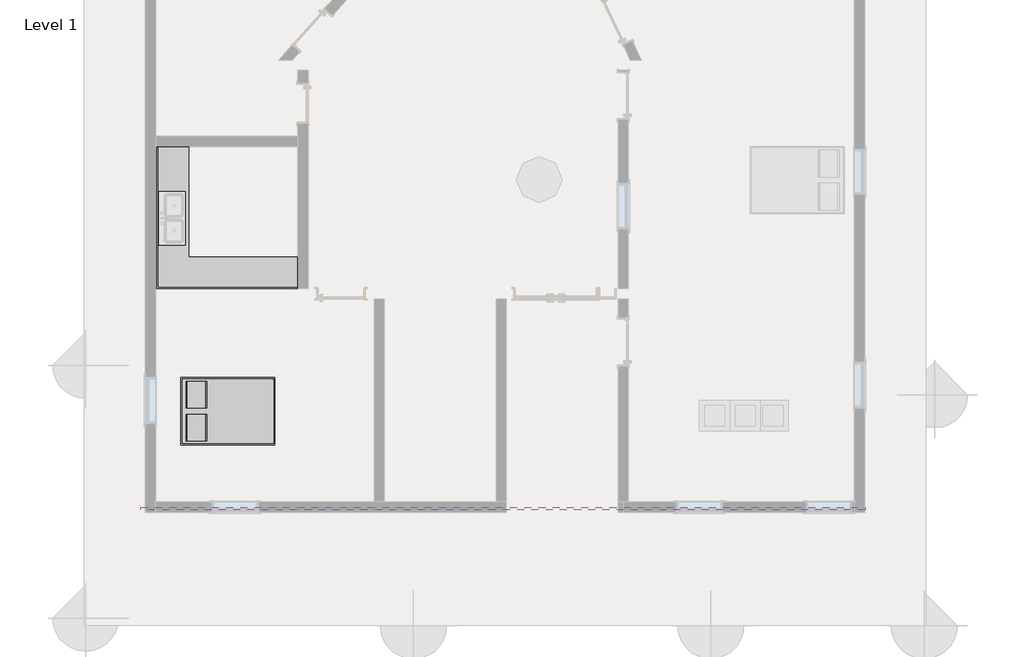
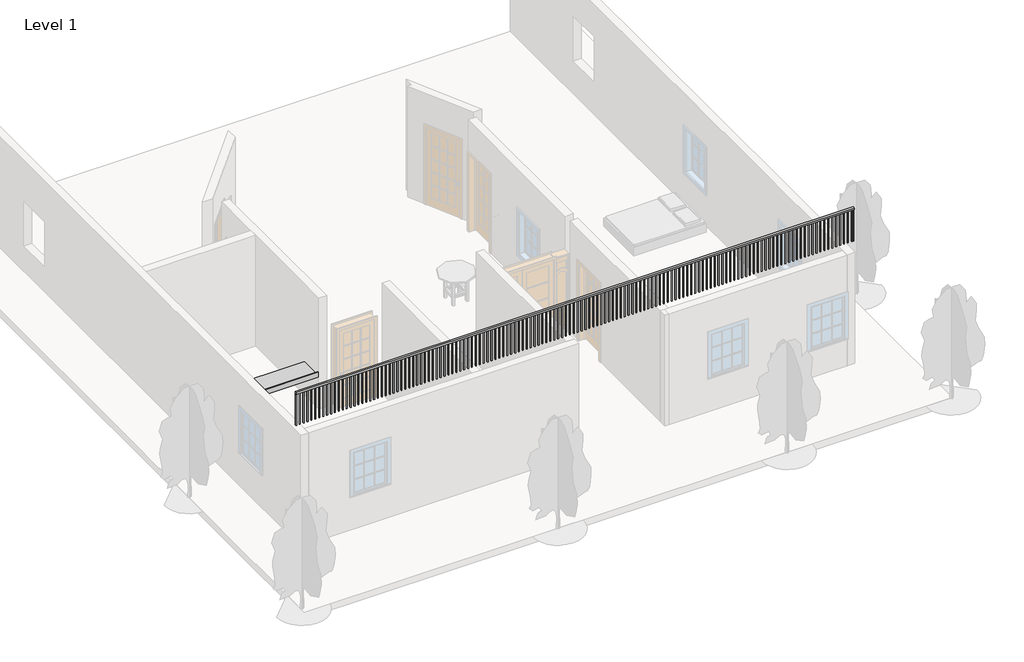
# One storey, part 2 of 3: 2 furniture elements, 1 railing.
"""IFC4 building model written with IfcOpenShell, lengths in millimetres."""

from ifc_helpers import new_model, si_unit, frame, origin, place, context, project, spatial, polyline, outline, extrude, transform, mapped, element, save
from components import furniture_c8abb964, furniture_ce44b9f3

model = new_model("IFC4")

# Units and contexts
model_context = context("Model", 3, world=origin())
ifc_project = project(units=[si_unit("LENGTHUNIT", "METRE", prefix="MILLI")], contexts=[model_context])

# Site, building, storey
site = spatial("IfcSite", under=ifc_project)
building = spatial("IfcBuilding", under=site)
storey = spatial("IfcBuildingStorey", under=building, Name="Level 1", Elevation=0.0)

# Furniture
placement = place(None, origin())
furniture_shape = furniture_c8abb964(model_context)
element("IfcFurniture", 1, ObjectType="Bed-Box : Double 53\" x 74\"", at=placement, inside=storey, context=model_context, shape_type="MappedRepresentation", body=[
    mapped(furniture_shape, transform((-8121.5392959, 5074.7783356, 0.0), x_axis=(0.0, 1.0000000000000018, 0.0), y_axis=(-1.0000000000000018, 0.0, 0.0), z_axis=(0.0, 0.0, 1.0))),
])
furniture_2_shape = furniture_ce44b9f3(model_context)
element("IfcFurniture", 2, ObjectType="Counter Top-L Shaped w Sink.0001 : 24\" Depth", at=placement, inside=storey, context=model_context, shape_type="MappedRepresentation", body=[
    mapped(furniture_2_shape, transform((-9309.5097877, 9065.4930897, 0.0), x_axis=(0.0, 1.0, 0.0), y_axis=(-1.0, 0.0, 0.0), z_axis=(0.0, 0.0, 1.0))),
])

# Railing
element("IfcRailing", 3, ObjectType="Handrail - Rectangular", at=placement, inside=storey, context=model_context, shape_type="SweptSolid", body=[
    extrude(outline(polyline([(-9630.8642944, 3438.5335491), (-9630.8642944, 3489.3335491), (4847.1357056, 3489.3335491), (4847.1357056, 3438.5335491), (-9630.8642944, 3438.5335491)])), frame((0.0, 0.0, 4185.9398438), z_axis=(0.0, 0.0, 1.0), x_axis=(1.0, 0.0, 0.0)), (0.0, 0.0, 1.0), 50.8),
    extrude(outline(polyline([(4786.8107056, 3454.4085491), (4786.8107056, 3473.4585491), (4805.8607056, 3473.4585491), (4805.8607056, 3454.4085491), (4786.8107056, 3454.4085491)])), frame((0.0, 0.0, 3322.3398438), z_axis=(0.0, 0.0, 1.0), x_axis=(1.0, 0.0, 0.0)), (0.0, 0.0, 1.0), 863.6),
    extrude(outline(polyline([(4685.2107056, 3454.4085491), (4685.2107056, 3473.4585491), (4704.2607056, 3473.4585491), (4704.2607056, 3454.4085491), (4685.2107056, 3454.4085491)])), frame((0.0, 0.0, 3322.3398438), z_axis=(0.0, 0.0, 1.0), x_axis=(1.0, 0.0, 0.0)), (0.0, 0.0, 1.0), 863.6),
    extrude(outline(polyline([(4583.6107056, 3454.4085491), (4583.6107056, 3473.4585491), (4602.6607056, 3473.4585491), (4602.6607056, 3454.4085491), (4583.6107056, 3454.4085491)])), frame((0.0, 0.0, 3322.3398438), z_axis=(0.0, 0.0, 1.0), x_axis=(1.0, 0.0, 0.0)), (0.0, 0.0, 1.0), 863.6),
    extrude(outline(polyline([(4482.0107056, 3454.4085491), (4482.0107056, 3473.4585491), (4501.0607056, 3473.4585491), (4501.0607056, 3454.4085491), (4482.0107056, 3454.4085491)])), frame((0.0, 0.0, 3322.3398438), z_axis=(0.0, 0.0, 1.0), x_axis=(1.0, 0.0, 0.0)), (0.0, 0.0, 1.0), 863.6),
    extrude(outline(polyline([(4380.4107056, 3454.4085491), (4380.4107056, 3473.4585491), (4399.4607056, 3473.4585491), (4399.4607056, 3454.4085491), (4380.4107056, 3454.4085491)])), frame((0.0, 0.0, 3322.3398438), z_axis=(0.0, 0.0, 1.0), x_axis=(1.0, 0.0, 0.0)), (0.0, 0.0, 1.0), 863.6),
    extrude(outline(polyline([(4278.8107056, 3454.4085491), (4278.8107056, 3473.4585491), (4297.8607056, 3473.4585491), (4297.8607056, 3454.4085491), (4278.8107056, 3454.4085491)])), frame((0.0, 0.0, 3322.3398438), z_axis=(0.0, 0.0, 1.0), x_axis=(1.0, 0.0, 0.0)), (0.0, 0.0, 1.0), 863.6),
    extrude(outline(polyline([(4177.2107056, 3454.4085491), (4177.2107056, 3473.4585491), (4196.2607056, 3473.4585491), (4196.2607056, 3454.4085491), (4177.2107056, 3454.4085491)])), frame((0.0, 0.0, 3322.3398438), z_axis=(0.0, 0.0, 1.0), x_axis=(1.0, 0.0, 0.0)), (0.0, 0.0, 1.0), 863.6),
    extrude(outline(polyline([(4075.6107056, 3454.4085491), (4075.6107056, 3473.4585491), (4094.6607056, 3473.4585491), (4094.6607056, 3454.4085491), (4075.6107056, 3454.4085491)])), frame((0.0, 0.0, 3322.3398438), z_axis=(0.0, 0.0, 1.0), x_axis=(1.0, 0.0, 0.0)), (0.0, 0.0, 1.0), 863.6),
    extrude(outline(polyline([(3974.0107056, 3454.4085491), (3974.0107056, 3473.4585491), (3993.0607056, 3473.4585491), (3993.0607056, 3454.4085491), (3974.0107056, 3454.4085491)])), frame((0.0, 0.0, 3322.3398438), z_axis=(0.0, 0.0, 1.0), x_axis=(1.0, 0.0, 0.0)), (0.0, 0.0, 1.0), 863.6),
    extrude(outline(polyline([(3872.4107056, 3454.4085491), (3872.4107056, 3473.4585491), (3891.4607056, 3473.4585491), (3891.4607056, 3454.4085491), (3872.4107056, 3454.4085491)])), frame((0.0, 0.0, 3322.3398438), z_axis=(0.0, 0.0, 1.0), x_axis=(1.0, 0.0, 0.0)), (0.0, 0.0, 1.0), 863.6),
    extrude(outline(polyline([(3770.8107056, 3454.4085491), (3770.8107056, 3473.4585491), (3789.8607056, 3473.4585491), (3789.8607056, 3454.4085491), (3770.8107056, 3454.4085491)])), frame((0.0, 0.0, 3322.3398438), z_axis=(0.0, 0.0, 1.0), x_axis=(1.0, 0.0, 0.0)), (0.0, 0.0, 1.0), 863.6),
    extrude(outline(polyline([(3669.2107056, 3454.4085491), (3669.2107056, 3473.4585491), (3688.2607056, 3473.4585491), (3688.2607056, 3454.4085491), (3669.2107056, 3454.4085491)])), frame((0.0, 0.0, 3322.3398438), z_axis=(0.0, 0.0, 1.0), x_axis=(1.0, 0.0, 0.0)), (0.0, 0.0, 1.0), 863.6),
    extrude(outline(polyline([(3567.6107056, 3454.4085491), (3567.6107056, 3473.4585491), (3586.6607056, 3473.4585491), (3586.6607056, 3454.4085491), (3567.6107056, 3454.4085491)])), frame((0.0, 0.0, 3322.3398438), z_axis=(0.0, 0.0, 1.0), x_axis=(1.0, 0.0, 0.0)), (0.0, 0.0, 1.0), 863.6),
    extrude(outline(polyline([(3466.0107056, 3454.4085491), (3466.0107056, 3473.4585491), (3485.0607056, 3473.4585491), (3485.0607056, 3454.4085491), (3466.0107056, 3454.4085491)])), frame((0.0, 0.0, 3322.3398438), z_axis=(0.0, 0.0, 1.0), x_axis=(1.0, 0.0, 0.0)), (0.0, 0.0, 1.0), 863.6),
    extrude(outline(polyline([(3364.4107056, 3454.4085491), (3364.4107056, 3473.4585491), (3383.4607056, 3473.4585491), (3383.4607056, 3454.4085491), (3364.4107056, 3454.4085491)])), frame((0.0, 0.0, 3322.3398438), z_axis=(0.0, 0.0, 1.0), x_axis=(1.0, 0.0, 0.0)), (0.0, 0.0, 1.0), 863.6),
    extrude(outline(polyline([(3262.8107056, 3454.4085491), (3262.8107056, 3473.4585491), (3281.8607056, 3473.4585491), (3281.8607056, 3454.4085491), (3262.8107056, 3454.4085491)])), frame((0.0, 0.0, 3322.3398438), z_axis=(0.0, 0.0, 1.0), x_axis=(1.0, 0.0, 0.0)), (0.0, 0.0, 1.0), 863.6),
    extrude(outline(polyline([(3161.2107056, 3454.4085491), (3161.2107056, 3473.4585491), (3180.2607056, 3473.4585491), (3180.2607056, 3454.4085491), (3161.2107056, 3454.4085491)])), frame((0.0, 0.0, 3322.3398438), z_axis=(0.0, 0.0, 1.0), x_axis=(1.0, 0.0, 0.0)), (0.0, 0.0, 1.0), 863.6),
    extrude(outline(polyline([(3059.6107056, 3454.4085491), (3059.6107056, 3473.4585491), (3078.6607056, 3473.4585491), (3078.6607056, 3454.4085491), (3059.6107056, 3454.4085491)])), frame((0.0, 0.0, 3322.3398438), z_axis=(0.0, 0.0, 1.0), x_axis=(1.0, 0.0, 0.0)), (0.0, 0.0, 1.0), 863.6),
    extrude(outline(polyline([(2958.0107056, 3454.4085491), (2958.0107056, 3473.4585491), (2977.0607056, 3473.4585491), (2977.0607056, 3454.4085491), (2958.0107056, 3454.4085491)])), frame((0.0, 0.0, 3322.3398438), z_axis=(0.0, 0.0, 1.0), x_axis=(1.0, 0.0, 0.0)), (0.0, 0.0, 1.0), 863.6),
    extrude(outline(polyline([(2856.4107056, 3454.4085491), (2856.4107056, 3473.4585491), (2875.4607056, 3473.4585491), (2875.4607056, 3454.4085491), (2856.4107056, 3454.4085491)])), frame((0.0, 0.0, 3322.3398438), z_axis=(0.0, 0.0, 1.0), x_axis=(1.0, 0.0, 0.0)), (0.0, 0.0, 1.0), 863.6),
    extrude(outline(polyline([(2754.8107056, 3454.4085491), (2754.8107056, 3473.4585491), (2773.8607056, 3473.4585491), (2773.8607056, 3454.4085491), (2754.8107056, 3454.4085491)])), frame((0.0, 0.0, 3322.3398438), z_axis=(0.0, 0.0, 1.0), x_axis=(1.0, 0.0, 0.0)), (0.0, 0.0, 1.0), 863.6),
    extrude(outline(polyline([(2653.2107056, 3454.4085491), (2653.2107056, 3473.4585491), (2672.2607056, 3473.4585491), (2672.2607056, 3454.4085491), (2653.2107056, 3454.4085491)])), frame((0.0, 0.0, 3322.3398438), z_axis=(0.0, 0.0, 1.0), x_axis=(1.0, 0.0, 0.0)), (0.0, 0.0, 1.0), 863.6),
    extrude(outline(polyline([(2551.6107056, 3454.4085491), (2551.6107056, 3473.4585491), (2570.6607056, 3473.4585491), (2570.6607056, 3454.4085491), (2551.6107056, 3454.4085491)])), frame((0.0, 0.0, 3322.3398438), z_axis=(0.0, 0.0, 1.0), x_axis=(1.0, 0.0, 0.0)), (0.0, 0.0, 1.0), 863.6),
    extrude(outline(polyline([(2450.0107056, 3454.4085491), (2450.0107056, 3473.4585491), (2469.0607056, 3473.4585491), (2469.0607056, 3454.4085491), (2450.0107056, 3454.4085491)])), frame((0.0, 0.0, 3322.3398438), z_axis=(0.0, 0.0, 1.0), x_axis=(1.0, 0.0, 0.0)), (0.0, 0.0, 1.0), 863.6),
    extrude(outline(polyline([(2348.4107056, 3454.4085491), (2348.4107056, 3473.4585491), (2367.4607056, 3473.4585491), (2367.4607056, 3454.4085491), (2348.4107056, 3454.4085491)])), frame((0.0, 0.0, 3322.3398438), z_axis=(0.0, 0.0, 1.0), x_axis=(1.0, 0.0, 0.0)), (0.0, 0.0, 1.0), 863.6),
    extrude(outline(polyline([(2246.8107056, 3454.4085491), (2246.8107056, 3473.4585491), (2265.8607056, 3473.4585491), (2265.8607056, 3454.4085491), (2246.8107056, 3454.4085491)])), frame((0.0, 0.0, 3322.3398438), z_axis=(0.0, 0.0, 1.0), x_axis=(1.0, 0.0, 0.0)), (0.0, 0.0, 1.0), 863.6),
    extrude(outline(polyline([(2145.2107056, 3454.4085491), (2145.2107056, 3473.4585491), (2164.2607056, 3473.4585491), (2164.2607056, 3454.4085491), (2145.2107056, 3454.4085491)])), frame((0.0, 0.0, 3322.3398438), z_axis=(0.0, 0.0, 1.0), x_axis=(1.0, 0.0, 0.0)), (0.0, 0.0, 1.0), 863.6),
    extrude(outline(polyline([(2043.6107056, 3454.4085491), (2043.6107056, 3473.4585491), (2062.6607056, 3473.4585491), (2062.6607056, 3454.4085491), (2043.6107056, 3454.4085491)])), frame((0.0, 0.0, 3322.3398438), z_axis=(0.0, 0.0, 1.0), x_axis=(1.0, 0.0, 0.0)), (0.0, 0.0, 1.0), 863.6),
    extrude(outline(polyline([(1942.0107056, 3454.4085491), (1942.0107056, 3473.4585491), (1961.0607056, 3473.4585491), (1961.0607056, 3454.4085491), (1942.0107056, 3454.4085491)])), frame((0.0, 0.0, 3322.3398438), z_axis=(0.0, 0.0, 1.0), x_axis=(1.0, 0.0, 0.0)), (0.0, 0.0, 1.0), 863.6),
    extrude(outline(polyline([(1840.4107056, 3454.4085491), (1840.4107056, 3473.4585491), (1859.4607056, 3473.4585491), (1859.4607056, 3454.4085491), (1840.4107056, 3454.4085491)])), frame((0.0, 0.0, 3322.3398438), z_axis=(0.0, 0.0, 1.0), x_axis=(1.0, 0.0, 0.0)), (0.0, 0.0, 1.0), 863.6),
    extrude(outline(polyline([(1738.8107056, 3454.4085491), (1738.8107056, 3473.4585491), (1757.8607056, 3473.4585491), (1757.8607056, 3454.4085491), (1738.8107056, 3454.4085491)])), frame((0.0, 0.0, 3322.3398438), z_axis=(0.0, 0.0, 1.0), x_axis=(1.0, 0.0, 0.0)), (0.0, 0.0, 1.0), 863.6),
    extrude(outline(polyline([(1637.2107056, 3454.4085491), (1637.2107056, 3473.4585491), (1656.2607056, 3473.4585491), (1656.2607056, 3454.4085491), (1637.2107056, 3454.4085491)])), frame((0.0, 0.0, 3322.3398438), z_axis=(0.0, 0.0, 1.0), x_axis=(1.0, 0.0, 0.0)), (0.0, 0.0, 1.0), 863.6),
    extrude(outline(polyline([(1535.6107056, 3454.4085491), (1535.6107056, 3473.4585491), (1554.6607056, 3473.4585491), (1554.6607056, 3454.4085491), (1535.6107056, 3454.4085491)])), frame((0.0, 0.0, 3322.3398438), z_axis=(0.0, 0.0, 1.0), x_axis=(1.0, 0.0, 0.0)), (0.0, 0.0, 1.0), 863.6),
    extrude(outline(polyline([(1434.0107056, 3454.4085491), (1434.0107056, 3473.4585491), (1453.0607056, 3473.4585491), (1453.0607056, 3454.4085491), (1434.0107056, 3454.4085491)])), frame((0.0, 0.0, 3322.3398438), z_axis=(0.0, 0.0, 1.0), x_axis=(1.0, 0.0, 0.0)), (0.0, 0.0, 1.0), 863.6),
    extrude(outline(polyline([(1332.4107056, 3454.4085491), (1332.4107056, 3473.4585491), (1351.4607056, 3473.4585491), (1351.4607056, 3454.4085491), (1332.4107056, 3454.4085491)])), frame((0.0, 0.0, 3322.3398438), z_axis=(0.0, 0.0, 1.0), x_axis=(1.0, 0.0, 0.0)), (0.0, 0.0, 1.0), 863.6),
    extrude(outline(polyline([(1230.8107056, 3454.4085491), (1230.8107056, 3473.4585491), (1249.8607056, 3473.4585491), (1249.8607056, 3454.4085491), (1230.8107056, 3454.4085491)])), frame((0.0, 0.0, 3322.3398438), z_axis=(0.0, 0.0, 1.0), x_axis=(1.0, 0.0, 0.0)), (0.0, 0.0, 1.0), 863.6),
    extrude(outline(polyline([(1129.2107056, 3454.4085491), (1129.2107056, 3473.4585491), (1148.2607056, 3473.4585491), (1148.2607056, 3454.4085491), (1129.2107056, 3454.4085491)])), frame((0.0, 0.0, 3322.3398438), z_axis=(0.0, 0.0, 1.0), x_axis=(1.0, 0.0, 0.0)), (0.0, 0.0, 1.0), 863.6),
    extrude(outline(polyline([(1027.6107056, 3454.4085491), (1027.6107056, 3473.4585491), (1046.6607056, 3473.4585491), (1046.6607056, 3454.4085491), (1027.6107056, 3454.4085491)])), frame((0.0, 0.0, 3322.3398438), z_axis=(0.0, 0.0, 1.0), x_axis=(1.0, 0.0, 0.0)), (0.0, 0.0, 1.0), 863.6),
    extrude(outline(polyline([(926.0107056, 3454.4085491), (926.0107056, 3473.4585491), (945.0607056, 3473.4585491), (945.0607056, 3454.4085491), (926.0107056, 3454.4085491)])), frame((0.0, 0.0, 3322.3398438), z_axis=(0.0, 0.0, 1.0), x_axis=(1.0, 0.0, 0.0)), (0.0, 0.0, 1.0), 863.6),
    extrude(outline(polyline([(824.4107056, 3454.4085491), (824.4107056, 3473.4585491), (843.4607056, 3473.4585491), (843.4607056, 3454.4085491), (824.4107056, 3454.4085491)])), frame((0.0, 0.0, 3322.3398438), z_axis=(0.0, 0.0, 1.0), x_axis=(1.0, 0.0, 0.0)), (0.0, 0.0, 1.0), 863.6),
    extrude(outline(polyline([(722.8107056, 3454.4085491), (722.8107056, 3473.4585491), (741.8607056, 3473.4585491), (741.8607056, 3454.4085491), (722.8107056, 3454.4085491)])), frame((0.0, 0.0, 3322.3398438), z_axis=(0.0, 0.0, 1.0), x_axis=(1.0, 0.0, 0.0)), (0.0, 0.0, 1.0), 863.6),
    extrude(outline(polyline([(621.2107056, 3454.4085491), (621.2107056, 3473.4585491), (640.2607056, 3473.4585491), (640.2607056, 3454.4085491), (621.2107056, 3454.4085491)])), frame((0.0, 0.0, 3322.3398438), z_axis=(0.0, 0.0, 1.0), x_axis=(1.0, 0.0, 0.0)), (0.0, 0.0, 1.0), 863.6),
    extrude(outline(polyline([(519.6107056, 3454.4085491), (519.6107056, 3473.4585491), (538.6607056, 3473.4585491), (538.6607056, 3454.4085491), (519.6107056, 3454.4085491)])), frame((0.0, 0.0, 3322.3398438), z_axis=(0.0, 0.0, 1.0), x_axis=(1.0, 0.0, 0.0)), (0.0, 0.0, 1.0), 863.6),
    extrude(outline(polyline([(418.0107056, 3454.4085491), (418.0107056, 3473.4585491), (437.0607056, 3473.4585491), (437.0607056, 3454.4085491), (418.0107056, 3454.4085491)])), frame((0.0, 0.0, 3322.3398438), z_axis=(0.0, 0.0, 1.0), x_axis=(1.0, 0.0, 0.0)), (0.0, 0.0, 1.0), 863.6),
    extrude(outline(polyline([(316.4107056, 3454.4085491), (316.4107056, 3473.4585491), (335.4607056, 3473.4585491), (335.4607056, 3454.4085491), (316.4107056, 3454.4085491)])), frame((0.0, 0.0, 3322.3398438), z_axis=(0.0, 0.0, 1.0), x_axis=(1.0, 0.0, 0.0)), (0.0, 0.0, 1.0), 863.6),
    extrude(outline(polyline([(214.8107056, 3454.4085491), (214.8107056, 3473.4585491), (233.8607056, 3473.4585491), (233.8607056, 3454.4085491), (214.8107056, 3454.4085491)])), frame((0.0, 0.0, 3322.3398438), z_axis=(0.0, 0.0, 1.0), x_axis=(1.0, 0.0, 0.0)), (0.0, 0.0, 1.0), 863.6),
    extrude(outline(polyline([(113.2107056, 3454.4085491), (113.2107056, 3473.4585491), (132.2607056, 3473.4585491), (132.2607056, 3454.4085491), (113.2107056, 3454.4085491)])), frame((0.0, 0.0, 3322.3398438), z_axis=(0.0, 0.0, 1.0), x_axis=(1.0, 0.0, 0.0)), (0.0, 0.0, 1.0), 863.6),
    extrude(outline(polyline([(11.6107056, 3454.4085491), (11.6107056, 3473.4585491), (30.6607056, 3473.4585491), (30.6607056, 3454.4085491), (11.6107056, 3454.4085491)])), frame((0.0, 0.0, 3322.3398438), z_axis=(0.0, 0.0, 1.0), x_axis=(1.0, 0.0, 0.0)), (0.0, 0.0, 1.0), 863.6),
    extrude(outline(polyline([(-89.9892944, 3454.4085491), (-89.9892944, 3473.4585491), (-70.9392944, 3473.4585491), (-70.9392944, 3454.4085491), (-89.9892944, 3454.4085491)])), frame((0.0, 0.0, 3322.3398438), z_axis=(0.0, 0.0, 1.0), x_axis=(1.0, 0.0, 0.0)), (0.0, 0.0, 1.0), 863.6),
    extrude(outline(polyline([(-191.5892944, 3454.4085491), (-191.5892944, 3473.4585491), (-172.5392944, 3473.4585491), (-172.5392944, 3454.4085491), (-191.5892944, 3454.4085491)])), frame((0.0, 0.0, 3322.3398438), z_axis=(0.0, 0.0, 1.0), x_axis=(1.0, 0.0, 0.0)), (0.0, 0.0, 1.0), 863.6),
    extrude(outline(polyline([(-293.1892944, 3454.4085491), (-293.1892944, 3473.4585491), (-274.1392944, 3473.4585491), (-274.1392944, 3454.4085491), (-293.1892944, 3454.4085491)])), frame((0.0, 0.0, 3322.3398438), z_axis=(0.0, 0.0, 1.0), x_axis=(1.0, 0.0, 0.0)), (0.0, 0.0, 1.0), 863.6),
    extrude(outline(polyline([(-394.7892944, 3454.4085491), (-394.7892944, 3473.4585491), (-375.7392944, 3473.4585491), (-375.7392944, 3454.4085491), (-394.7892944, 3454.4085491)])), frame((0.0, 0.0, 3322.3398438), z_axis=(0.0, 0.0, 1.0), x_axis=(1.0, 0.0, 0.0)), (0.0, 0.0, 1.0), 863.6),
    extrude(outline(polyline([(-496.3892944, 3454.4085491), (-496.3892944, 3473.4585491), (-477.3392944, 3473.4585491), (-477.3392944, 3454.4085491), (-496.3892944, 3454.4085491)])), frame((0.0, 0.0, 3322.3398438), z_axis=(0.0, 0.0, 1.0), x_axis=(1.0, 0.0, 0.0)), (0.0, 0.0, 1.0), 863.6),
    extrude(outline(polyline([(-597.9892944, 3454.4085491), (-597.9892944, 3473.4585491), (-578.9392944, 3473.4585491), (-578.9392944, 3454.4085491), (-597.9892944, 3454.4085491)])), frame((0.0, 0.0, 3322.3398438), z_axis=(0.0, 0.0, 1.0), x_axis=(1.0, 0.0, 0.0)), (0.0, 0.0, 1.0), 863.6),
    extrude(outline(polyline([(-699.5892944, 3454.4085491), (-699.5892944, 3473.4585491), (-680.5392944, 3473.4585491), (-680.5392944, 3454.4085491), (-699.5892944, 3454.4085491)])), frame((0.0, 0.0, 3322.3398438), z_axis=(0.0, 0.0, 1.0), x_axis=(1.0, 0.0, 0.0)), (0.0, 0.0, 1.0), 863.6),
    extrude(outline(polyline([(-801.1892944, 3454.4085491), (-801.1892944, 3473.4585491), (-782.1392944, 3473.4585491), (-782.1392944, 3454.4085491), (-801.1892944, 3454.4085491)])), frame((0.0, 0.0, 3322.3398438), z_axis=(0.0, 0.0, 1.0), x_axis=(1.0, 0.0, 0.0)), (0.0, 0.0, 1.0), 863.6),
    extrude(outline(polyline([(-902.7892944, 3454.4085491), (-902.7892944, 3473.4585491), (-883.7392944, 3473.4585491), (-883.7392944, 3454.4085491), (-902.7892944, 3454.4085491)])), frame((0.0, 0.0, 3322.3398438), z_axis=(0.0, 0.0, 1.0), x_axis=(1.0, 0.0, 0.0)), (0.0, 0.0, 1.0), 863.6),
    extrude(outline(polyline([(-1004.3892944, 3454.4085491), (-1004.3892944, 3473.4585491), (-985.3392944, 3473.4585491), (-985.3392944, 3454.4085491), (-1004.3892944, 3454.4085491)])), frame((0.0, 0.0, 3322.3398438), z_axis=(0.0, 0.0, 1.0), x_axis=(1.0, 0.0, 0.0)), (0.0, 0.0, 1.0), 863.6),
    extrude(outline(polyline([(-1105.9892944, 3454.4085491), (-1105.9892944, 3473.4585491), (-1086.9392944, 3473.4585491), (-1086.9392944, 3454.4085491), (-1105.9892944, 3454.4085491)])), frame((0.0, 0.0, 3322.3398438), z_axis=(0.0, 0.0, 1.0), x_axis=(1.0, 0.0, 0.0)), (0.0, 0.0, 1.0), 863.6),
    extrude(outline(polyline([(-1207.5892944, 3454.4085491), (-1207.5892944, 3473.4585491), (-1188.5392944, 3473.4585491), (-1188.5392944, 3454.4085491), (-1207.5892944, 3454.4085491)])), frame((0.0, 0.0, 3322.3398438), z_axis=(0.0, 0.0, 1.0), x_axis=(1.0, 0.0, 0.0)), (0.0, 0.0, 1.0), 863.6),
    extrude(outline(polyline([(-1309.1892944, 3454.4085491), (-1309.1892944, 3473.4585491), (-1290.1392944, 3473.4585491), (-1290.1392944, 3454.4085491), (-1309.1892944, 3454.4085491)])), frame((0.0, 0.0, 3322.3398438), z_axis=(0.0, 0.0, 1.0), x_axis=(1.0, 0.0, 0.0)), (0.0, 0.0, 1.0), 863.6),
    extrude(outline(polyline([(-1410.7892944, 3454.4085491), (-1410.7892944, 3473.4585491), (-1391.7392944, 3473.4585491), (-1391.7392944, 3454.4085491), (-1410.7892944, 3454.4085491)])), frame((0.0, 0.0, 3322.3398438), z_axis=(0.0, 0.0, 1.0), x_axis=(1.0, 0.0, 0.0)), (0.0, 0.0, 1.0), 863.6),
    extrude(outline(polyline([(-1512.3892944, 3454.4085491), (-1512.3892944, 3473.4585491), (-1493.3392944, 3473.4585491), (-1493.3392944, 3454.4085491), (-1512.3892944, 3454.4085491)])), frame((0.0, 0.0, 3322.3398438), z_axis=(0.0, 0.0, 1.0), x_axis=(1.0, 0.0, 0.0)), (0.0, 0.0, 1.0), 863.6),
    extrude(outline(polyline([(-1613.9892944, 3454.4085491), (-1613.9892944, 3473.4585491), (-1594.9392944, 3473.4585491), (-1594.9392944, 3454.4085491), (-1613.9892944, 3454.4085491)])), frame((0.0, 0.0, 3322.3398438), z_axis=(0.0, 0.0, 1.0), x_axis=(1.0, 0.0, 0.0)), (0.0, 0.0, 1.0), 863.6),
    extrude(outline(polyline([(-1715.5892944, 3454.4085491), (-1715.5892944, 3473.4585491), (-1696.5392944, 3473.4585491), (-1696.5392944, 3454.4085491), (-1715.5892944, 3454.4085491)])), frame((0.0, 0.0, 3322.3398438), z_axis=(0.0, 0.0, 1.0), x_axis=(1.0, 0.0, 0.0)), (0.0, 0.0, 1.0), 863.6),
    extrude(outline(polyline([(-1817.1892944, 3454.4085491), (-1817.1892944, 3473.4585491), (-1798.1392944, 3473.4585491), (-1798.1392944, 3454.4085491), (-1817.1892944, 3454.4085491)])), frame((0.0, 0.0, 3322.3398438), z_axis=(0.0, 0.0, 1.0), x_axis=(1.0, 0.0, 0.0)), (0.0, 0.0, 1.0), 863.6),
    extrude(outline(polyline([(-1918.7892944, 3454.4085491), (-1918.7892944, 3473.4585491), (-1899.7392944, 3473.4585491), (-1899.7392944, 3454.4085491), (-1918.7892944, 3454.4085491)])), frame((0.0, 0.0, 3322.3398438), z_axis=(0.0, 0.0, 1.0), x_axis=(1.0, 0.0, 0.0)), (0.0, 0.0, 1.0), 863.6),
    extrude(outline(polyline([(-2020.3892944, 3454.4085491), (-2020.3892944, 3473.4585491), (-2001.3392944, 3473.4585491), (-2001.3392944, 3454.4085491), (-2020.3892944, 3454.4085491)])), frame((0.0, 0.0, 3322.3398438), z_axis=(0.0, 0.0, 1.0), x_axis=(1.0, 0.0, 0.0)), (0.0, 0.0, 1.0), 863.6),
    extrude(outline(polyline([(-2121.9892944, 3454.4085491), (-2121.9892944, 3473.4585491), (-2102.9392944, 3473.4585491), (-2102.9392944, 3454.4085491), (-2121.9892944, 3454.4085491)])), frame((0.0, 0.0, 3322.3398438), z_axis=(0.0, 0.0, 1.0), x_axis=(1.0, 0.0, 0.0)), (0.0, 0.0, 1.0), 863.6),
    extrude(outline(polyline([(-2223.5892944, 3454.4085491), (-2223.5892944, 3473.4585491), (-2204.5392944, 3473.4585491), (-2204.5392944, 3454.4085491), (-2223.5892944, 3454.4085491)])), frame((0.0, 0.0, 3322.3398438), z_axis=(0.0, 0.0, 1.0), x_axis=(1.0, 0.0, 0.0)), (0.0, 0.0, 1.0), 863.6),
    extrude(outline(polyline([(-2325.1892944, 3454.4085491), (-2325.1892944, 3473.4585491), (-2306.1392944, 3473.4585491), (-2306.1392944, 3454.4085491), (-2325.1892944, 3454.4085491)])), frame((0.0, 0.0, 3322.3398438), z_axis=(0.0, 0.0, 1.0), x_axis=(1.0, 0.0, 0.0)), (0.0, 0.0, 1.0), 863.6),
    extrude(outline(polyline([(-2426.7892944, 3454.4085491), (-2426.7892944, 3473.4585491), (-2407.7392944, 3473.4585491), (-2407.7392944, 3454.4085491), (-2426.7892944, 3454.4085491)])), frame((0.0, 0.0, 3322.3398438), z_axis=(0.0, 0.0, 1.0), x_axis=(1.0, 0.0, 0.0)), (0.0, 0.0, 1.0), 863.6),
    extrude(outline(polyline([(-2528.3892944, 3454.4085491), (-2528.3892944, 3473.4585491), (-2509.3392944, 3473.4585491), (-2509.3392944, 3454.4085491), (-2528.3892944, 3454.4085491)])), frame((0.0, 0.0, 3322.3398438), z_axis=(0.0, 0.0, 1.0), x_axis=(1.0, 0.0, 0.0)), (0.0, 0.0, 1.0), 863.6),
    extrude(outline(polyline([(-2629.9892944, 3454.4085491), (-2629.9892944, 3473.4585491), (-2610.9392944, 3473.4585491), (-2610.9392944, 3454.4085491), (-2629.9892944, 3454.4085491)])), frame((0.0, 0.0, 3322.3398438), z_axis=(0.0, 0.0, 1.0), x_axis=(1.0, 0.0, 0.0)), (0.0, 0.0, 1.0), 863.6),
    extrude(outline(polyline([(-2731.5892944, 3454.4085491), (-2731.5892944, 3473.4585491), (-2712.5392944, 3473.4585491), (-2712.5392944, 3454.4085491), (-2731.5892944, 3454.4085491)])), frame((0.0, 0.0, 3322.3398438), z_axis=(0.0, 0.0, 1.0), x_axis=(1.0, 0.0, 0.0)), (0.0, 0.0, 1.0), 863.6),
    extrude(outline(polyline([(-2833.1892944, 3454.4085491), (-2833.1892944, 3473.4585491), (-2814.1392944, 3473.4585491), (-2814.1392944, 3454.4085491), (-2833.1892944, 3454.4085491)])), frame((0.0, 0.0, 3322.3398438), z_axis=(0.0, 0.0, 1.0), x_axis=(1.0, 0.0, 0.0)), (0.0, 0.0, 1.0), 863.6),
    extrude(outline(polyline([(-2934.7892944, 3454.4085491), (-2934.7892944, 3473.4585491), (-2915.7392944, 3473.4585491), (-2915.7392944, 3454.4085491), (-2934.7892944, 3454.4085491)])), frame((0.0, 0.0, 3322.3398438), z_axis=(0.0, 0.0, 1.0), x_axis=(1.0, 0.0, 0.0)), (0.0, 0.0, 1.0), 863.6),
    extrude(outline(polyline([(-3036.3892944, 3454.4085491), (-3036.3892944, 3473.4585491), (-3017.3392944, 3473.4585491), (-3017.3392944, 3454.4085491), (-3036.3892944, 3454.4085491)])), frame((0.0, 0.0, 3322.3398438), z_axis=(0.0, 0.0, 1.0), x_axis=(1.0, 0.0, 0.0)), (0.0, 0.0, 1.0), 863.6),
    extrude(outline(polyline([(-3137.9892944, 3454.4085491), (-3137.9892944, 3473.4585491), (-3118.9392944, 3473.4585491), (-3118.9392944, 3454.4085491), (-3137.9892944, 3454.4085491)])), frame((0.0, 0.0, 3322.3398438), z_axis=(0.0, 0.0, 1.0), x_axis=(1.0, 0.0, 0.0)), (0.0, 0.0, 1.0), 863.6),
    extrude(outline(polyline([(-3239.5892944, 3454.4085491), (-3239.5892944, 3473.4585491), (-3220.5392944, 3473.4585491), (-3220.5392944, 3454.4085491), (-3239.5892944, 3454.4085491)])), frame((0.0, 0.0, 3322.3398438), z_axis=(0.0, 0.0, 1.0), x_axis=(1.0, 0.0, 0.0)), (0.0, 0.0, 1.0), 863.6),
    extrude(outline(polyline([(-3341.1892944, 3454.4085491), (-3341.1892944, 3473.4585491), (-3322.1392944, 3473.4585491), (-3322.1392944, 3454.4085491), (-3341.1892944, 3454.4085491)])), frame((0.0, 0.0, 3322.3398438), z_axis=(0.0, 0.0, 1.0), x_axis=(1.0, 0.0, 0.0)), (0.0, 0.0, 1.0), 863.6),
    extrude(outline(polyline([(-3442.7892944, 3454.4085491), (-3442.7892944, 3473.4585491), (-3423.7392944, 3473.4585491), (-3423.7392944, 3454.4085491), (-3442.7892944, 3454.4085491)])), frame((0.0, 0.0, 3322.3398438), z_axis=(0.0, 0.0, 1.0), x_axis=(1.0, 0.0, 0.0)), (0.0, 0.0, 1.0), 863.6),
    extrude(outline(polyline([(-3544.3892944, 3454.4085491), (-3544.3892944, 3473.4585491), (-3525.3392944, 3473.4585491), (-3525.3392944, 3454.4085491), (-3544.3892944, 3454.4085491)])), frame((0.0, 0.0, 3322.3398438), z_axis=(0.0, 0.0, 1.0), x_axis=(1.0, 0.0, 0.0)), (0.0, 0.0, 1.0), 863.6),
    extrude(outline(polyline([(-3645.9892944, 3454.4085491), (-3645.9892944, 3473.4585491), (-3626.9392944, 3473.4585491), (-3626.9392944, 3454.4085491), (-3645.9892944, 3454.4085491)])), frame((0.0, 0.0, 3322.3398438), z_axis=(0.0, 0.0, 1.0), x_axis=(1.0, 0.0, 0.0)), (0.0, 0.0, 1.0), 863.6),
    extrude(outline(polyline([(-3747.5892944, 3454.4085491), (-3747.5892944, 3473.4585491), (-3728.5392944, 3473.4585491), (-3728.5392944, 3454.4085491), (-3747.5892944, 3454.4085491)])), frame((0.0, 0.0, 3322.3398438), z_axis=(0.0, 0.0, 1.0), x_axis=(1.0, 0.0, 0.0)), (0.0, 0.0, 1.0), 863.6),
    extrude(outline(polyline([(-3849.1892944, 3454.4085491), (-3849.1892944, 3473.4585491), (-3830.1392944, 3473.4585491), (-3830.1392944, 3454.4085491), (-3849.1892944, 3454.4085491)])), frame((0.0, 0.0, 3322.3398438), z_axis=(0.0, 0.0, 1.0), x_axis=(1.0, 0.0, 0.0)), (0.0, 0.0, 1.0), 863.6),
    extrude(outline(polyline([(-3950.7892944, 3454.4085491), (-3950.7892944, 3473.4585491), (-3931.7392944, 3473.4585491), (-3931.7392944, 3454.4085491), (-3950.7892944, 3454.4085491)])), frame((0.0, 0.0, 3322.3398438), z_axis=(0.0, 0.0, 1.0), x_axis=(1.0, 0.0, 0.0)), (0.0, 0.0, 1.0), 863.6),
    extrude(outline(polyline([(-4052.3892944, 3454.4085491), (-4052.3892944, 3473.4585491), (-4033.3392944, 3473.4585491), (-4033.3392944, 3454.4085491), (-4052.3892944, 3454.4085491)])), frame((0.0, 0.0, 3322.3398438), z_axis=(0.0, 0.0, 1.0), x_axis=(1.0, 0.0, 0.0)), (0.0, 0.0, 1.0), 863.6),
    extrude(outline(polyline([(-4153.9892944, 3454.4085491), (-4153.9892944, 3473.4585491), (-4134.9392944, 3473.4585491), (-4134.9392944, 3454.4085491), (-4153.9892944, 3454.4085491)])), frame((0.0, 0.0, 3322.3398438), z_axis=(0.0, 0.0, 1.0), x_axis=(1.0, 0.0, 0.0)), (0.0, 0.0, 1.0), 863.6),
    extrude(outline(polyline([(-4255.5892944, 3454.4085491), (-4255.5892944, 3473.4585491), (-4236.5392944, 3473.4585491), (-4236.5392944, 3454.4085491), (-4255.5892944, 3454.4085491)])), frame((0.0, 0.0, 3322.3398438), z_axis=(0.0, 0.0, 1.0), x_axis=(1.0, 0.0, 0.0)), (0.0, 0.0, 1.0), 863.6),
    extrude(outline(polyline([(-4357.1892944, 3454.4085491), (-4357.1892944, 3473.4585491), (-4338.1392944, 3473.4585491), (-4338.1392944, 3454.4085491), (-4357.1892944, 3454.4085491)])), frame((0.0, 0.0, 3322.3398438), z_axis=(0.0, 0.0, 1.0), x_axis=(1.0, 0.0, 0.0)), (0.0, 0.0, 1.0), 863.6),
    extrude(outline(polyline([(-4458.7892944, 3454.4085491), (-4458.7892944, 3473.4585491), (-4439.7392944, 3473.4585491), (-4439.7392944, 3454.4085491), (-4458.7892944, 3454.4085491)])), frame((0.0, 0.0, 3322.3398438), z_axis=(0.0, 0.0, 1.0), x_axis=(1.0, 0.0, 0.0)), (0.0, 0.0, 1.0), 863.6),
    extrude(outline(polyline([(-4560.3892944, 3454.4085491), (-4560.3892944, 3473.4585491), (-4541.3392944, 3473.4585491), (-4541.3392944, 3454.4085491), (-4560.3892944, 3454.4085491)])), frame((0.0, 0.0, 3322.3398438), z_axis=(0.0, 0.0, 1.0), x_axis=(1.0, 0.0, 0.0)), (0.0, 0.0, 1.0), 863.6),
    extrude(outline(polyline([(-4661.9892944, 3454.4085491), (-4661.9892944, 3473.4585491), (-4642.9392944, 3473.4585491), (-4642.9392944, 3454.4085491), (-4661.9892944, 3454.4085491)])), frame((0.0, 0.0, 3322.3398438), z_axis=(0.0, 0.0, 1.0), x_axis=(1.0, 0.0, 0.0)), (0.0, 0.0, 1.0), 863.6),
    extrude(outline(polyline([(-4763.5892944, 3454.4085491), (-4763.5892944, 3473.4585491), (-4744.5392944, 3473.4585491), (-4744.5392944, 3454.4085491), (-4763.5892944, 3454.4085491)])), frame((0.0, 0.0, 3322.3398438), z_axis=(0.0, 0.0, 1.0), x_axis=(1.0, 0.0, 0.0)), (0.0, 0.0, 1.0), 863.6),
    extrude(outline(polyline([(-4865.1892944, 3454.4085491), (-4865.1892944, 3473.4585491), (-4846.1392944, 3473.4585491), (-4846.1392944, 3454.4085491), (-4865.1892944, 3454.4085491)])), frame((0.0, 0.0, 3322.3398438), z_axis=(0.0, 0.0, 1.0), x_axis=(1.0, 0.0, 0.0)), (0.0, 0.0, 1.0), 863.6),
    extrude(outline(polyline([(-4966.7892944, 3454.4085491), (-4966.7892944, 3473.4585491), (-4947.7392944, 3473.4585491), (-4947.7392944, 3454.4085491), (-4966.7892944, 3454.4085491)])), frame((0.0, 0.0, 3322.3398438), z_axis=(0.0, 0.0, 1.0), x_axis=(1.0, 0.0, 0.0)), (0.0, 0.0, 1.0), 863.6),
    extrude(outline(polyline([(-5068.3892944, 3454.4085491), (-5068.3892944, 3473.4585491), (-5049.3392944, 3473.4585491), (-5049.3392944, 3454.4085491), (-5068.3892944, 3454.4085491)])), frame((0.0, 0.0, 3322.3398438), z_axis=(0.0, 0.0, 1.0), x_axis=(1.0, 0.0, 0.0)), (0.0, 0.0, 1.0), 863.6),
    extrude(outline(polyline([(-5169.9892944, 3454.4085491), (-5169.9892944, 3473.4585491), (-5150.9392944, 3473.4585491), (-5150.9392944, 3454.4085491), (-5169.9892944, 3454.4085491)])), frame((0.0, 0.0, 3322.3398438), z_axis=(0.0, 0.0, 1.0), x_axis=(1.0, 0.0, 0.0)), (0.0, 0.0, 1.0), 863.6),
    extrude(outline(polyline([(-5271.5892944, 3454.4085491), (-5271.5892944, 3473.4585491), (-5252.5392944, 3473.4585491), (-5252.5392944, 3454.4085491), (-5271.5892944, 3454.4085491)])), frame((0.0, 0.0, 3322.3398438), z_axis=(0.0, 0.0, 1.0), x_axis=(1.0, 0.0, 0.0)), (0.0, 0.0, 1.0), 863.6),
    extrude(outline(polyline([(-5373.1892944, 3454.4085491), (-5373.1892944, 3473.4585491), (-5354.1392944, 3473.4585491), (-5354.1392944, 3454.4085491), (-5373.1892944, 3454.4085491)])), frame((0.0, 0.0, 3322.3398438), z_axis=(0.0, 0.0, 1.0), x_axis=(1.0, 0.0, 0.0)), (0.0, 0.0, 1.0), 863.6),
    extrude(outline(polyline([(-5474.7892944, 3454.4085491), (-5474.7892944, 3473.4585491), (-5455.7392944, 3473.4585491), (-5455.7392944, 3454.4085491), (-5474.7892944, 3454.4085491)])), frame((0.0, 0.0, 3322.3398438), z_axis=(0.0, 0.0, 1.0), x_axis=(1.0, 0.0, 0.0)), (0.0, 0.0, 1.0), 863.6),
    extrude(outline(polyline([(-5576.3892944, 3454.4085491), (-5576.3892944, 3473.4585491), (-5557.3392944, 3473.4585491), (-5557.3392944, 3454.4085491), (-5576.3892944, 3454.4085491)])), frame((0.0, 0.0, 3322.3398438), z_axis=(0.0, 0.0, 1.0), x_axis=(1.0, 0.0, 0.0)), (0.0, 0.0, 1.0), 863.6),
    extrude(outline(polyline([(-5677.9892944, 3454.4085491), (-5677.9892944, 3473.4585491), (-5658.9392944, 3473.4585491), (-5658.9392944, 3454.4085491), (-5677.9892944, 3454.4085491)])), frame((0.0, 0.0, 3322.3398438), z_axis=(0.0, 0.0, 1.0), x_axis=(1.0, 0.0, 0.0)), (0.0, 0.0, 1.0), 863.6),
    extrude(outline(polyline([(-5779.5892944, 3454.4085491), (-5779.5892944, 3473.4585491), (-5760.5392944, 3473.4585491), (-5760.5392944, 3454.4085491), (-5779.5892944, 3454.4085491)])), frame((0.0, 0.0, 3322.3398438), z_axis=(0.0, 0.0, 1.0), x_axis=(1.0, 0.0, 0.0)), (0.0, 0.0, 1.0), 863.6),
    extrude(outline(polyline([(-5881.1892944, 3454.4085491), (-5881.1892944, 3473.4585491), (-5862.1392944, 3473.4585491), (-5862.1392944, 3454.4085491), (-5881.1892944, 3454.4085491)])), frame((0.0, 0.0, 3322.3398438), z_axis=(0.0, 0.0, 1.0), x_axis=(1.0, 0.0, 0.0)), (0.0, 0.0, 1.0), 863.6),
    extrude(outline(polyline([(-5982.7892944, 3454.4085491), (-5982.7892944, 3473.4585491), (-5963.7392944, 3473.4585491), (-5963.7392944, 3454.4085491), (-5982.7892944, 3454.4085491)])), frame((0.0, 0.0, 3322.3398438), z_axis=(0.0, 0.0, 1.0), x_axis=(1.0, 0.0, 0.0)), (0.0, 0.0, 1.0), 863.6),
    extrude(outline(polyline([(-6084.3892944, 3454.4085491), (-6084.3892944, 3473.4585491), (-6065.3392944, 3473.4585491), (-6065.3392944, 3454.4085491), (-6084.3892944, 3454.4085491)])), frame((0.0, 0.0, 3322.3398438), z_axis=(0.0, 0.0, 1.0), x_axis=(1.0, 0.0, 0.0)), (0.0, 0.0, 1.0), 863.6),
    extrude(outline(polyline([(-6185.9892944, 3454.4085491), (-6185.9892944, 3473.4585491), (-6166.9392944, 3473.4585491), (-6166.9392944, 3454.4085491), (-6185.9892944, 3454.4085491)])), frame((0.0, 0.0, 3322.3398438), z_axis=(0.0, 0.0, 1.0), x_axis=(1.0, 0.0, 0.0)), (0.0, 0.0, 1.0), 863.6),
    extrude(outline(polyline([(-6287.5892944, 3454.4085491), (-6287.5892944, 3473.4585491), (-6268.5392944, 3473.4585491), (-6268.5392944, 3454.4085491), (-6287.5892944, 3454.4085491)])), frame((0.0, 0.0, 3322.3398438), z_axis=(0.0, 0.0, 1.0), x_axis=(1.0, 0.0, 0.0)), (0.0, 0.0, 1.0), 863.6),
    extrude(outline(polyline([(-6389.1892944, 3454.4085491), (-6389.1892944, 3473.4585491), (-6370.1392944, 3473.4585491), (-6370.1392944, 3454.4085491), (-6389.1892944, 3454.4085491)])), frame((0.0, 0.0, 3322.3398438), z_axis=(0.0, 0.0, 1.0), x_axis=(1.0, 0.0, 0.0)), (0.0, 0.0, 1.0), 863.6),
    extrude(outline(polyline([(-6490.7892944, 3454.4085491), (-6490.7892944, 3473.4585491), (-6471.7392944, 3473.4585491), (-6471.7392944, 3454.4085491), (-6490.7892944, 3454.4085491)])), frame((0.0, 0.0, 3322.3398438), z_axis=(0.0, 0.0, 1.0), x_axis=(1.0, 0.0, 0.0)), (0.0, 0.0, 1.0), 863.6),
    extrude(outline(polyline([(-6592.3892944, 3454.4085491), (-6592.3892944, 3473.4585491), (-6573.3392944, 3473.4585491), (-6573.3392944, 3454.4085491), (-6592.3892944, 3454.4085491)])), frame((0.0, 0.0, 3322.3398438), z_axis=(0.0, 0.0, 1.0), x_axis=(1.0, 0.0, 0.0)), (0.0, 0.0, 1.0), 863.6),
    extrude(outline(polyline([(-6693.9892944, 3454.4085491), (-6693.9892944, 3473.4585491), (-6674.9392944, 3473.4585491), (-6674.9392944, 3454.4085491), (-6693.9892944, 3454.4085491)])), frame((0.0, 0.0, 3322.3398438), z_axis=(0.0, 0.0, 1.0), x_axis=(1.0, 0.0, 0.0)), (0.0, 0.0, 1.0), 863.6),
    extrude(outline(polyline([(-6795.5892944, 3454.4085491), (-6795.5892944, 3473.4585491), (-6776.5392944, 3473.4585491), (-6776.5392944, 3454.4085491), (-6795.5892944, 3454.4085491)])), frame((0.0, 0.0, 3322.3398438), z_axis=(0.0, 0.0, 1.0), x_axis=(1.0, 0.0, 0.0)), (0.0, 0.0, 1.0), 863.6),
    extrude(outline(polyline([(-6897.1892944, 3454.4085491), (-6897.1892944, 3473.4585491), (-6878.1392944, 3473.4585491), (-6878.1392944, 3454.4085491), (-6897.1892944, 3454.4085491)])), frame((0.0, 0.0, 3322.3398438), z_axis=(0.0, 0.0, 1.0), x_axis=(1.0, 0.0, 0.0)), (0.0, 0.0, 1.0), 863.6),
    extrude(outline(polyline([(-6998.7892944, 3454.4085491), (-6998.7892944, 3473.4585491), (-6979.7392944, 3473.4585491), (-6979.7392944, 3454.4085491), (-6998.7892944, 3454.4085491)])), frame((0.0, 0.0, 3322.3398438), z_axis=(0.0, 0.0, 1.0), x_axis=(1.0, 0.0, 0.0)), (0.0, 0.0, 1.0), 863.6),
    extrude(outline(polyline([(-7100.3892944, 3454.4085491), (-7100.3892944, 3473.4585491), (-7081.3392944, 3473.4585491), (-7081.3392944, 3454.4085491), (-7100.3892944, 3454.4085491)])), frame((0.0, 0.0, 3322.3398438), z_axis=(0.0, 0.0, 1.0), x_axis=(1.0, 0.0, 0.0)), (0.0, 0.0, 1.0), 863.6),
    extrude(outline(polyline([(-7201.9892944, 3454.4085491), (-7201.9892944, 3473.4585491), (-7182.9392944, 3473.4585491), (-7182.9392944, 3454.4085491), (-7201.9892944, 3454.4085491)])), frame((0.0, 0.0, 3322.3398438), z_axis=(0.0, 0.0, 1.0), x_axis=(1.0, 0.0, 0.0)), (0.0, 0.0, 1.0), 863.6),
    extrude(outline(polyline([(-7303.5892944, 3454.4085491), (-7303.5892944, 3473.4585491), (-7284.5392944, 3473.4585491), (-7284.5392944, 3454.4085491), (-7303.5892944, 3454.4085491)])), frame((0.0, 0.0, 3322.3398438), z_axis=(0.0, 0.0, 1.0), x_axis=(1.0, 0.0, 0.0)), (0.0, 0.0, 1.0), 863.6),
    extrude(outline(polyline([(-7405.1892944, 3454.4085491), (-7405.1892944, 3473.4585491), (-7386.1392944, 3473.4585491), (-7386.1392944, 3454.4085491), (-7405.1892944, 3454.4085491)])), frame((0.0, 0.0, 3322.3398438), z_axis=(0.0, 0.0, 1.0), x_axis=(1.0, 0.0, 0.0)), (0.0, 0.0, 1.0), 863.6),
    extrude(outline(polyline([(-7506.7892944, 3454.4085491), (-7506.7892944, 3473.4585491), (-7487.7392944, 3473.4585491), (-7487.7392944, 3454.4085491), (-7506.7892944, 3454.4085491)])), frame((0.0, 0.0, 3322.3398438), z_axis=(0.0, 0.0, 1.0), x_axis=(1.0, 0.0, 0.0)), (0.0, 0.0, 1.0), 863.6),
    extrude(outline(polyline([(-7608.3892944, 3454.4085491), (-7608.3892944, 3473.4585491), (-7589.3392944, 3473.4585491), (-7589.3392944, 3454.4085491), (-7608.3892944, 3454.4085491)])), frame((0.0, 0.0, 3322.3398438), z_axis=(0.0, 0.0, 1.0), x_axis=(1.0, 0.0, 0.0)), (0.0, 0.0, 1.0), 863.6),
    extrude(outline(polyline([(-7709.9892944, 3454.4085491), (-7709.9892944, 3473.4585491), (-7690.9392944, 3473.4585491), (-7690.9392944, 3454.4085491), (-7709.9892944, 3454.4085491)])), frame((0.0, 0.0, 3322.3398438), z_axis=(0.0, 0.0, 1.0), x_axis=(1.0, 0.0, 0.0)), (0.0, 0.0, 1.0), 863.6),
    extrude(outline(polyline([(-7811.5892944, 3454.4085491), (-7811.5892944, 3473.4585491), (-7792.5392944, 3473.4585491), (-7792.5392944, 3454.4085491), (-7811.5892944, 3454.4085491)])), frame((0.0, 0.0, 3322.3398438), z_axis=(0.0, 0.0, 1.0), x_axis=(1.0, 0.0, 0.0)), (0.0, 0.0, 1.0), 863.6),
    extrude(outline(polyline([(-7913.1892944, 3454.4085491), (-7913.1892944, 3473.4585491), (-7894.1392944, 3473.4585491), (-7894.1392944, 3454.4085491), (-7913.1892944, 3454.4085491)])), frame((0.0, 0.0, 3322.3398438), z_axis=(0.0, 0.0, 1.0), x_axis=(1.0, 0.0, 0.0)), (0.0, 0.0, 1.0), 863.6),
    extrude(outline(polyline([(-8014.7892944, 3454.4085491), (-8014.7892944, 3473.4585491), (-7995.7392944, 3473.4585491), (-7995.7392944, 3454.4085491), (-8014.7892944, 3454.4085491)])), frame((0.0, 0.0, 3322.3398438), z_axis=(0.0, 0.0, 1.0), x_axis=(1.0, 0.0, 0.0)), (0.0, 0.0, 1.0), 863.6),
    extrude(outline(polyline([(-8116.3892944, 3454.4085491), (-8116.3892944, 3473.4585491), (-8097.3392944, 3473.4585491), (-8097.3392944, 3454.4085491), (-8116.3892944, 3454.4085491)])), frame((0.0, 0.0, 3322.3398438), z_axis=(0.0, 0.0, 1.0), x_axis=(1.0, 0.0, 0.0)), (0.0, 0.0, 1.0), 863.6),
    extrude(outline(polyline([(-8217.9892944, 3454.4085491), (-8217.9892944, 3473.4585491), (-8198.9392944, 3473.4585491), (-8198.9392944, 3454.4085491), (-8217.9892944, 3454.4085491)])), frame((0.0, 0.0, 3322.3398438), z_axis=(0.0, 0.0, 1.0), x_axis=(1.0, 0.0, 0.0)), (0.0, 0.0, 1.0), 863.6),
    extrude(outline(polyline([(-8319.5892944, 3454.4085491), (-8319.5892944, 3473.4585491), (-8300.5392944, 3473.4585491), (-8300.5392944, 3454.4085491), (-8319.5892944, 3454.4085491)])), frame((0.0, 0.0, 3322.3398438), z_axis=(0.0, 0.0, 1.0), x_axis=(1.0, 0.0, 0.0)), (0.0, 0.0, 1.0), 863.6),
    extrude(outline(polyline([(-8421.1892944, 3454.4085491), (-8421.1892944, 3473.4585491), (-8402.1392944, 3473.4585491), (-8402.1392944, 3454.4085491), (-8421.1892944, 3454.4085491)])), frame((0.0, 0.0, 3322.3398438), z_axis=(0.0, 0.0, 1.0), x_axis=(1.0, 0.0, 0.0)), (0.0, 0.0, 1.0), 863.6),
    extrude(outline(polyline([(-8522.7892944, 3454.4085491), (-8522.7892944, 3473.4585491), (-8503.7392944, 3473.4585491), (-8503.7392944, 3454.4085491), (-8522.7892944, 3454.4085491)])), frame((0.0, 0.0, 3322.3398438), z_axis=(0.0, 0.0, 1.0), x_axis=(1.0, 0.0, 0.0)), (0.0, 0.0, 1.0), 863.6),
    extrude(outline(polyline([(-8624.3892944, 3454.4085491), (-8624.3892944, 3473.4585491), (-8605.3392944, 3473.4585491), (-8605.3392944, 3454.4085491), (-8624.3892944, 3454.4085491)])), frame((0.0, 0.0, 3322.3398438), z_axis=(0.0, 0.0, 1.0), x_axis=(1.0, 0.0, 0.0)), (0.0, 0.0, 1.0), 863.6),
    extrude(outline(polyline([(-8725.9892944, 3454.4085491), (-8725.9892944, 3473.4585491), (-8706.9392944, 3473.4585491), (-8706.9392944, 3454.4085491), (-8725.9892944, 3454.4085491)])), frame((0.0, 0.0, 3322.3398438), z_axis=(0.0, 0.0, 1.0), x_axis=(1.0, 0.0, 0.0)), (0.0, 0.0, 1.0), 863.6),
    extrude(outline(polyline([(-8827.5892944, 3454.4085491), (-8827.5892944, 3473.4585491), (-8808.5392944, 3473.4585491), (-8808.5392944, 3454.4085491), (-8827.5892944, 3454.4085491)])), frame((0.0, 0.0, 3322.3398438), z_axis=(0.0, 0.0, 1.0), x_axis=(1.0, 0.0, 0.0)), (0.0, 0.0, 1.0), 863.6),
    extrude(outline(polyline([(-8929.1892944, 3454.4085491), (-8929.1892944, 3473.4585491), (-8910.1392944, 3473.4585491), (-8910.1392944, 3454.4085491), (-8929.1892944, 3454.4085491)])), frame((0.0, 0.0, 3322.3398438), z_axis=(0.0, 0.0, 1.0), x_axis=(1.0, 0.0, 0.0)), (0.0, 0.0, 1.0), 863.6),
    extrude(outline(polyline([(-9030.7892944, 3454.4085491), (-9030.7892944, 3473.4585491), (-9011.7392944, 3473.4585491), (-9011.7392944, 3454.4085491), (-9030.7892944, 3454.4085491)])), frame((0.0, 0.0, 3322.3398438), z_axis=(0.0, 0.0, 1.0), x_axis=(1.0, 0.0, 0.0)), (0.0, 0.0, 1.0), 863.6),
    extrude(outline(polyline([(-9132.3892944, 3454.4085491), (-9132.3892944, 3473.4585491), (-9113.3392944, 3473.4585491), (-9113.3392944, 3454.4085491), (-9132.3892944, 3454.4085491)])), frame((0.0, 0.0, 3322.3398438), z_axis=(0.0, 0.0, 1.0), x_axis=(1.0, 0.0, 0.0)), (0.0, 0.0, 1.0), 863.6),
    extrude(outline(polyline([(-9233.9892944, 3454.4085491), (-9233.9892944, 3473.4585491), (-9214.9392944, 3473.4585491), (-9214.9392944, 3454.4085491), (-9233.9892944, 3454.4085491)])), frame((0.0, 0.0, 3322.3398438), z_axis=(0.0, 0.0, 1.0), x_axis=(1.0, 0.0, 0.0)), (0.0, 0.0, 1.0), 863.6),
    extrude(outline(polyline([(-9335.5892944, 3454.4085491), (-9335.5892944, 3473.4585491), (-9316.5392944, 3473.4585491), (-9316.5392944, 3454.4085491), (-9335.5892944, 3454.4085491)])), frame((0.0, 0.0, 3322.3398438), z_axis=(0.0, 0.0, 1.0), x_axis=(1.0, 0.0, 0.0)), (0.0, 0.0, 1.0), 863.6),
    extrude(outline(polyline([(-9437.1892944, 3454.4085491), (-9437.1892944, 3473.4585491), (-9418.1392944, 3473.4585491), (-9418.1392944, 3454.4085491), (-9437.1892944, 3454.4085491)])), frame((0.0, 0.0, 3322.3398438), z_axis=(0.0, 0.0, 1.0), x_axis=(1.0, 0.0, 0.0)), (0.0, 0.0, 1.0), 863.6),
    extrude(outline(polyline([(-9538.7892944, 3454.4085491), (-9538.7892944, 3473.4585491), (-9519.7392944, 3473.4585491), (-9519.7392944, 3454.4085491), (-9538.7892944, 3454.4085491)])), frame((0.0, 0.0, 3322.3398438), z_axis=(0.0, 0.0, 1.0), x_axis=(1.0, 0.0, 0.0)), (0.0, 0.0, 1.0), 863.6),
    extrude(outline(polyline([(4828.0857056, 3454.4085491), (4828.0857056, 3473.4585491), (4847.1357056, 3473.4585491), (4847.1357056, 3454.4085491), (4828.0857056, 3454.4085491)])), frame((0.0, 0.0, 3322.3398438), z_axis=(0.0, 0.0, 1.0), x_axis=(1.0, 0.0, 0.0)), (0.0, 0.0, 1.0), 863.6),
    extrude(outline(polyline([(-9630.8642944, 3454.4085491), (-9630.8642944, 3473.4585491), (-9611.8142944, 3473.4585491), (-9611.8142944, 3454.4085491), (-9630.8642944, 3454.4085491)])), frame((0.0, 0.0, 3322.3398438), z_axis=(0.0, 0.0, 1.0), x_axis=(1.0, 0.0, 0.0)), (0.0, 0.0, 1.0), 863.6),
])

save(model, "model.ifc")

# Revit data of these elements
# Type "Bed-Box : Double 53\" x 74\""
#   Assembly Code = "E2020200"
#   Length = 6' - 2"
#   Width = 4' - 5"
#   Frame Material = Birch
#   Mattress Material = Linen, White
#   Default Elevation = 0
# Type "Counter Top-L Shaped w Sink.0001 : 24\" Depth"
#   Assembly Code = "C1030400"
#   Counter Thickness = 0' - 1 1/2"
#   Depth = 2' - 1"
#   Height = 3' - 0"
#   Length - Leg 1 [instance default] = 8' - 0"
#   Length - Leg 2 [instance default] = 6' - 0"
#   Sink Location [instance default] = 3' - 0"
#   Sink Location To Wall [instance default] = 0' - 6"
#   Sink Opening Depth [instance default] = 1' - 3"
#   Sink Opening Width [instance default] = 3' - 3"
#   Counter Top Material = none
#   Default Elevation = 0
# Type "Handrail - Rectangular"
#   Assembly Code = "C2010400"
#   built-in parameter 1008612 = 0.0416667 (stored number, unit not read)
#   built-in parameter 1008611 = 0.0416667 (stored number, unit not read)
#   built-in parameter 1008609 = 0.333333 (stored number, unit not read)
#   built-in parameter 1008604 = 0.166667 (stored number, unit not read)
#   built-in parameter 1008603 = 0.166667 (stored number, unit not read)
#   Railing Height = 3' - 0"
#   built-in parameter 1008630 = 2
#   built-in parameter 1008610 = 2
#   built-in parameter 1008618 = Baluster - Square : 3/4"
# Element 1 (IfcFurniture, "Bed-Box : Double 53\" x 74\"")
#   Phase Created = New Construction
#   Materials on its faces: "Birch", "Linen, White"
# Element 2 (IfcFurniture, "Counter Top-L Shaped w Sink.0001 : 24\" Depth")
#   Sink Opening Width = 3' - 3"
#   Sink Opening Depth = 1' - 3"
#   Sink Location To Wall = 0' - 6"
#   Sink Location = 3' - 0"
#   Length - Leg 2 = 9' - 3"
#   Length - Leg 1 = 9' - 4"
#   Phase Created = New Construction
#   Materials on its faces: "Counter Top"
# Element 3 (IfcRailing, "Handrail - Rectangular")
#   built-in parameter 1008621 = 10.9001 (stored number, unit not read)
#   Phase Created = New Construction
# Materials
#   "Birch": class "Wood", colour RGB 224 178 126, transparency 0, Description = "Betula Alleghaniensis", Cost = 0
#   "Linen, White": class "Textile", colour RGB 247 247 239, transparency 0, Description = "Linen, white", Cost = 0
#   "Counter Top": class "Wood", colour RGB 226 177 128, transparency 0
